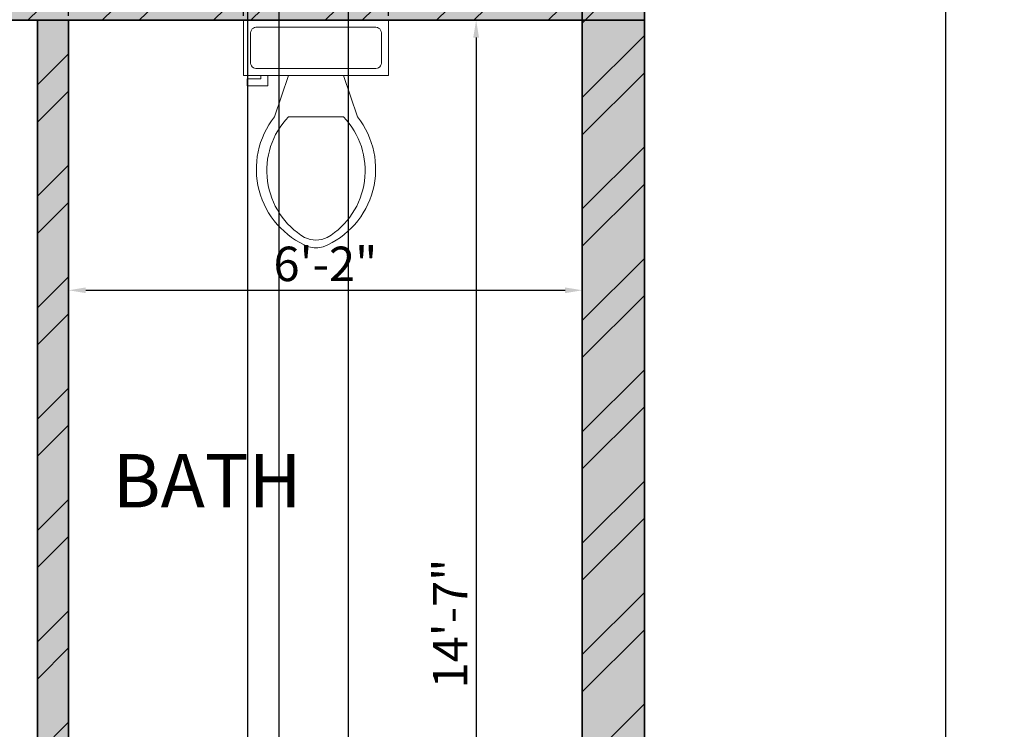
# Model space of a CAD drawing. Units: inches. Extents: x 1804 to 3296, y 909 to 2477.
# Tile 17 of 31: x 2235 to 2378, y 1484 to 1587. Entities that reach past the tile are written whole.
import ezdxf

# ---------------------------------------------------------------- set-up
doc = ezdxf.new("R2010")
doc.units = ezdxf.units.IN
for name, color, linetype, lineweight in [('A-ANNO-DIMS', 2, 'Continuous', 18), ('A-ANNO-TTLB', 156, 'Continuous', 35), ('A-AREA-IDEN', 190, 'Continuous', 18), ('A-FLOR-FIXT', 9, 'Continuous', 18), ('A-WALL-PATT', 10, 'Continuous', 13), ('WALL', 10, 'Continuous', 35)]:
    doc.layers.add(name, color=color, linetype=linetype, lineweight=lineweight)
doc.styles.get("Standard").update_dxf_attribs({"font": 'arial.ttf'})
doc.dimstyles.new('ISO-25', dxfattribs={"dimtxt": 5, "dimasz": 2.5, "dimexe": 1.25, "dimexo": 0.625, "dimtad": 1, "dimdec": 0, "dimlunit": 4, "dimtxsty": 'Standard', "dimcen": 2.5, "dimadec": 0, "dimazin": 0, "dimtfac": 1, "dimtdec": 0, "dimtmove": 0, "dimatfit": 3, "dimfxl": 1, "dimarcsym": 0})
pattern_1 = [(45, (0, 196.207), (-8.08223, 8.08223), []), (45, (5.388, 196.207), (-8.08223, 8.08223), [])]

# ---------------------------------------------------------------- blocks, each defined once
blk = doc.blocks.new('*U4')
for p, q in [((9.5, -6), (9.5, -2)), ((-10, -8.5), (-8, -8.5)), ((-10, -9.5), (-10, -8.5)), ((-8, -8.5), (-8, -8)), ((-7, -8), (-7, -9.5)), ((-4, -8), (-6, -14)), ((4, -8), (6, -14)), ((-7, -9.5), (-10, -9.5)), ((4, -14), (-4, -14))]:
    blk.add_line(p, q)
blk.add_lwpolyline([(10.5, -8), (10.5, 0), (-10.5, 0), (-10.5, -8)], close=True)
for points in [[(8.5, -1), (-8.5, -1)], [(-9.5, -2), (-9.5, -6)], [(-8.5, -7), (8.5, -7)]]:
    blk.add_lwpolyline(points)
for centre, radius, start, end in [((-8.62, -1.88), 0.884, 81.8699, 188.1301), ((8.62, -1.88), 0.884, 351.8699, 98.1301), ((-8.62, -6.12), 0.884, 171.8699, 278.1301), ((8.62, -6.12), 0.884, 261.8699, 8.1301), ((3.52, -21.58), 12.17, 141.4691, 247.9714), ((4.2, -21.82), 11.33, 136.3677, 238.9468), ((-3.52, -21.58), 12.17, 292.0284, 38.5307), ((-4.2, -21.82), 11.33, 301.053, 43.6321), ((0, -27.88), 4, 245.7318, 294.2682), ((0, -29), 4, 254.8605, 285.1395)]:
    blk.add_arc(centre, radius, start, end)
blk = doc.blocks.new('*D12')
at = {"layer": 'A-ANNO-DIMS', "color": 0, "lineweight": -2, "transparency": 16777216}
for p, q in [((2242.06, 1585.8), (2242.06, 1546)), ((2316.54, 1585.8), (2316.54, 1546)), ((2244.56, 1547.25), (2314.04, 1547.25))]:
    blk.add_line(p, q, dxfattribs=at)
at = {"layer": 'A-ANNO-DIMS', "color": 0, "lineweight": 100, "transparency": 16777216}
for points in [[(2244.56, 1547.66), (2244.56, 1546.83), (2242.06, 1547.25)], [(2314.04, 1547.66), (2314.04, 1546.83), (2316.54, 1547.25)]]:
    blk.add_solid(points, dxfattribs=at)
at = {"layer": 'Defpoints', "color": 0, "lineweight": 100, "transparency": 16777216}
for p in [(2242.06, 1586.42), (2316.54, 1586.42), (2316.54, 1547.25)]:
    blk.add_point(p, dxfattribs=at)
at = {"layer": 'A-ANNO-DIMS', "color": 0, "transparency": 16777216, "insert": (2279.3, 1550.43), "char_height": 5, "attachment_point": 5}
blk.add_mtext('6\'-2"', dxfattribs=at)
blk = doc.blocks.new('*D13')
at = {"layer": 'A-ANNO-DIMS', "color": 0, "lineweight": -2, "transparency": 16777216}
for p, q in [((2315.91, 1586.42), (2299.9, 1586.42)), ((2301.15, 1583.92), (2301.15, 1413.85)), ((2315.91, 1411.35), (2299.9, 1411.35))]:
    blk.add_line(p, q, dxfattribs=at)
at = {"layer": 'A-ANNO-DIMS', "color": 0, "lineweight": 100, "transparency": 16777216}
for points in [[(2300.73, 1583.92), (2301.57, 1583.92), (2301.15, 1586.42)], [(2300.73, 1413.85), (2301.57, 1413.85), (2301.15, 1411.35)]]:
    blk.add_solid(points, dxfattribs=at)
at = {"layer": 'Defpoints', "color": 0, "lineweight": 100, "transparency": 16777216}
for p in [(2316.54, 1586.42), (2301.15, 1411.35), (2316.54, 1411.35)]:
    blk.add_point(p, dxfattribs=at)
at = {"layer": 'A-ANNO-DIMS', "color": 0, "transparency": 16777216, "insert": (2298.02, 1498.89), "char_height": 5, "attachment_point": 5, "rotation": 90}
blk.add_mtext('14\'-7"', dxfattribs=at)
blk = doc.blocks.new('*D53')
at = {"layer": 'A-ANNO-DIMS', "color": 0, "lineweight": -2, "transparency": 16777216}
for p, q in [((2326.16, 1793.38), (2370.49, 1793.38)), ((2369.24, 1140.57), (2369.24, 1790.88)), ((2326.16, 1138.07), (2370.49, 1138.07))]:
    blk.add_line(p, q, dxfattribs=at)
at = {"layer": 'A-ANNO-DIMS', "color": 0, "lineweight": 100, "transparency": 16777216}
for points in [[(2368.82, 1790.88), (2369.65, 1790.88), (2369.24, 1793.38)], [(2368.82, 1140.57), (2369.65, 1140.57), (2369.24, 1138.07)]]:
    blk.add_solid(points, dxfattribs=at)
at = {"layer": 'Defpoints', "color": 0, "lineweight": 100, "transparency": 16777216}
for p in [(2325.54, 1793.38), (2369.24, 1793.38), (2325.54, 1138.07)]:
    blk.add_point(p, dxfattribs=at)
at = {"layer": 'A-ANNO-DIMS', "color": 0, "transparency": 16777216, "insert": (2366.03, 1465.72), "char_height": 5, "attachment_point": 5, "rotation": 90}
blk.add_mtext('54\'-7 1/2"', dxfattribs=at)
blk = doc.blocks.new('*D56')
at = {"layer": 'A-ANNO-DIMS', "color": 0, "lineweight": -2, "transparency": 16777216}
for p, q in [((2180.87, 1680.42), (2180.87, 975.89)), ((2268, 1680.42), (2268, 975.89)), ((2183.37, 977.14), (2265.5, 977.14))]:
    blk.add_line(p, q, dxfattribs=at)
at = {"layer": 'A-ANNO-DIMS', "color": 0, "lineweight": 100, "transparency": 16777216}
for points in [[(2183.37, 977.56), (2183.37, 976.72), (2180.87, 977.14)], [(2265.5, 977.56), (2265.5, 976.72), (2268, 977.14)]]:
    blk.add_solid(points, dxfattribs=at)
at = {"layer": 'Defpoints', "color": 0, "lineweight": 100, "transparency": 16777216}
for p in [(2180.87, 1681.04), (2268, 1681.04), (2268, 977.14)]:
    blk.add_point(p, dxfattribs=at)
at = {"layer": 'A-ANNO-DIMS', "color": 0, "transparency": 16777216, "insert": (2224.44, 980.32), "char_height": 5, "attachment_point": 5}
blk.add_mtext('7\'-3"', dxfattribs=at)
blk = doc.blocks.new('*D65')
at = {"layer": 'A-ANNO-DIMS', "color": 0, "lineweight": -2, "transparency": 16777216}
for p, q in [((2282.65, 1466.57), (2282.65, 1874.99)), ((2316.54, 1466.57), (2316.54, 1874.99)), ((2285.15, 1873.74), (2314.04, 1873.74))]:
    blk.add_line(p, q, dxfattribs=at)
at = {"layer": 'A-ANNO-DIMS', "color": 0, "lineweight": 100, "transparency": 16777216}
for points in [[(2285.15, 1874.15), (2285.15, 1873.32), (2282.65, 1873.74)], [(2314.04, 1874.15), (2314.04, 1873.32), (2316.54, 1873.74)]]:
    blk.add_solid(points, dxfattribs=at)
at = {"layer": 'Defpoints', "color": 0, "lineweight": 100, "transparency": 16777216}
for p in [(2316.54, 1873.74), (2282.65, 1465.94), (2316.54, 1465.94)]:
    blk.add_point(p, dxfattribs=at)
at = {"layer": 'A-ANNO-DIMS', "color": 0, "transparency": 16777216, "insert": (2299.6, 1876.91), "char_height": 5, "attachment_point": 5}
blk.add_mtext('2\'-10"', dxfattribs=at)
blk = doc.blocks.new('*D67')
at = {"layer": 'A-ANNO-DIMS', "color": 0, "lineweight": -2, "transparency": 16777216}
for p, q in [((2267.43, 1587.05), (2267.43, 1874.99)), ((2288.43, 1587.05), (2288.43, 1874.99)), ((2269.93, 1873.74), (2285.93, 1873.74))]:
    blk.add_line(p, q, dxfattribs=at)
at = {"layer": 'A-ANNO-DIMS', "color": 0, "lineweight": 100, "transparency": 16777216}
for points in [[(2269.93, 1874.15), (2269.93, 1873.32), (2267.43, 1873.74)], [(2285.93, 1874.15), (2285.93, 1873.32), (2288.43, 1873.74)]]:
    blk.add_solid(points, dxfattribs=at)
at = {"layer": 'Defpoints', "color": 0, "lineweight": 100, "transparency": 16777216}
for p in [(2288.43, 1873.74), (2267.43, 1586.42), (2288.43, 1586.42)]:
    blk.add_point(p, dxfattribs=at)
at = {"layer": 'A-ANNO-DIMS', "color": 0, "transparency": 16777216, "insert": (2277.93, 1876.91), "char_height": 5, "attachment_point": 5}
blk.add_mtext('1\'-9"', dxfattribs=at)
blk = doc.blocks.new('*D68')
at = {"layer": 'A-ANNO-DIMS', "color": 0, "lineweight": -2, "transparency": 16777216}
for p, q in [((2242.06, 1587.05), (2242.06, 1874.99)), ((2267.43, 1587.05), (2267.43, 1874.99)), ((2244.56, 1873.74), (2264.93, 1873.74)), ((2267.43, 1873.74), (2296.2, 1873.74))]:
    blk.add_line(p, q, dxfattribs=at)
at = {"layer": 'A-ANNO-DIMS', "color": 0, "lineweight": 100, "transparency": 16777216}
for points in [[(2244.56, 1874.15), (2244.56, 1873.32), (2242.06, 1873.74)], [(2264.93, 1874.15), (2264.93, 1873.32), (2267.43, 1873.74)]]:
    blk.add_solid(points, dxfattribs=at)
at = {"layer": 'Defpoints', "color": 0, "lineweight": 100, "transparency": 16777216}
for p in [(2267.43, 1873.74), (2242.06, 1586.42), (2267.43, 1586.42)]:
    blk.add_point(p, dxfattribs=at)
at = {"layer": 'A-ANNO-DIMS', "color": 0, "transparency": 16777216, "insert": (2283.07, 1876.95), "char_height": 5, "attachment_point": 5}
blk.add_mtext('2\'-1 1/2"', dxfattribs=at)
blk = doc.blocks.new('*D73')
at = {"layer": 'A-ANNO-DIMS', "color": 0, "lineweight": -2, "transparency": 16777216}
for p, q in [((2272.59, 1272.26), (2272.59, 1874.99)), ((2316.54, 1272.26), (2316.54, 1874.99)), ((2275.09, 1873.74), (2314.04, 1873.74))]:
    blk.add_line(p, q, dxfattribs=at)
at = {"layer": 'A-ANNO-DIMS', "color": 0, "lineweight": 100, "transparency": 16777216}
for points in [[(2275.09, 1874.15), (2275.09, 1873.32), (2272.59, 1873.74)], [(2314.04, 1874.15), (2314.04, 1873.32), (2316.54, 1873.74)]]:
    blk.add_solid(points, dxfattribs=at)
at = {"layer": 'Defpoints', "color": 0, "lineweight": 100, "transparency": 16777216}
for p in [(2316.54, 1873.74), (2272.59, 1271.63), (2316.54, 1271.63)]:
    blk.add_point(p, dxfattribs=at)
at = {"layer": 'A-ANNO-DIMS', "color": 0, "transparency": 16777216, "insert": (2294.56, 1876.92), "char_height": 5, "attachment_point": 5}
blk.add_mtext('3\'-8"', dxfattribs=at)

msp = doc.modelspace()

# ---------------------------------------------------------------- hatches: boundary and pattern name
at = {"layer": 'A-ANNO-TTLB'}
h = msp.add_hatch(color=256, dxfattribs=at)
h.dxf.hatch_style = 1
h.paths.add_polyline_path([(3294.53, 2476.54), (1803.79, 2476.54), (1805.43, 909.47), (3296.17, 909.47)])
h.paths.add_polyline_path([(1811, 914.33), (1812.79, 2467.54), (3285.53, 2467.54), (3283.74, 914.33)], flags=16)
h.paths.add_polyline_path([(1925.58, 1062.77), (1925.58, 1138.07), (1925.58, 1539.88), (1925.58, 1793.38), (1925.58, 1830.04), (2325.54, 1830.04), (2325.54, 1793.38), (2325.54, 1586.42), (2325.54, 1138.07), (2325.54, 1062.77)], flags=0)
h.paths.add_polyline_path([(1997.22, 1029.4), (2008.85, 1037.96), (2008.85, 1020.84)], flags=0)
h.paths.add_polyline_path([(1934.58, 1138.07), (1934.58, 1147.07), (2078.77, 1147.07), (2078.77, 1138.07), (2060.94, 1138.07)], flags=0)
h.paths.add_polyline_path([(1944.35, 1138.07), (1944.35, 1147.07), (2056.05, 1147.07), (2056.05, 1138.07)], flags=0)
h.paths.add_polyline_path([(2222.24, 1037.96), (2233.87, 1029.4), (2222.24, 1020.84)], flags=0)
h.paths.add_polyline_path([(2061.94, 1139.07), (2061.94, 1146.07), (2077.77, 1146.07), (2077.77, 1139.07)], flags=0)
h.paths.add_polyline_path([(2149.58, 1138.07), (2149.58, 1269.44), (2158.58, 1269.44), (2158.58, 1326.69), (2149.58, 1326.69), (2149.58, 1340.94), (2139.6, 1340.94), (2139.6, 1434.25), (2149.58, 1434.25), (2149.58, 1447.36), (2158.58, 1447.36), (2158.58, 1423.87), (2158.58, 1408.06), (2198.46, 1408.06), (2198.46, 1412.56), (2282.65, 1412.56), (2282.65, 1465.94), (2316.54, 1465.94), (2316.54, 1590.92), (2192.86, 1590.92), (2192.86, 1595.3), (2291.17, 1595.3), (2291.17, 1590.92), (2316.54, 1590.92), (2316.54, 1784.38), (2300.24, 1784.38), (2300.24, 1757.47), (2268, 1757.47), (2268, 1681.04), (2180.87, 1681.04), (2180.87, 1757.47), (2148.63, 1757.47), (2148.63, 1784.38), (2119.08, 1784.38), (2119.08, 1585.58), (2114.58, 1585.58), (2114.58, 1784.38), (2064.11, 1784.38), (2046.28, 1784.38), (2046.28, 1760.38), (1958.58, 1760.38), (1958.58, 1664.38), (1934.58, 1664.38), (1934.58, 1784.38), (1934.58, 1793.38), (2046.28, 1793.38), (2064.11, 1793.38), (2119.08, 1793.38), (2230.78, 1793.38), (2230.78, 1784.38), (2268, 1784.38), (2300.24, 1784.38), (2316.54, 1784.38), (2316.54, 1590.92), (2316.54, 1373.73), (2316.54, 1138.07)], flags=0)
h.paths.add_polyline_path([(2209.19, 1166.63), (2209.19, 1175.63), (2158.58, 1175.63), (2209.19, 1223.63), (2209.19, 1231.63), (2183.88, 1231.63), (2183.88, 1301.66), (2242.59, 1301.66), (2242.59, 1326.69), (2316.54, 1326.69), (2272.59, 1271.63), (2272.59, 1223.63), (2316.54, 1175.63), (2272.59, 1175.63), (2272.59, 1166.63)], flags=0)
h.paths.add_polyline_path([(1947.77, 1345.22), (1947.77, 1457.48), (1991.2, 1457.48), (1991.2, 1451.7), (1991.2, 1352.18), (1991.2, 1345.22)], flags=0)
h.paths.add_polyline_path([(2209.19, 1271.63), (2262.59, 1271.63), (2262.59, 1311.85), (2272.59, 1301.66), (2272.59, 1271.63), (2269.92, 1269.63), (2270.59, 1269.63), (2270.59, 1225.63), (2211.19, 1225.63), (2211.19, 1269.63), (2211.86, 1269.63)], flags=0)
h.paths.add_polyline_path([(2000.34, 1378.21), (2000.34, 1429.71), (2025.22, 1429.71), (2025.22, 1378.21)], flags=0)
h.paths.add_polyline_path([(2001.34, 1379.21), (2001.34, 1428.71), (2024.22, 1428.71), (2024.22, 1379.21)], flags=0)
h.paths.add_polyline_path([(2012.34, 1390.21), (2012.34, 1417.71), (2013.22, 1417.71), (2013.22, 1390.21)], flags=0)
h.paths.add_polyline_path([(2237.56, 1331.19), (2237.56, 1340.18), (2238.62, 1340.18), (2238.62, 1386.84), (2241.04, 1386.84), (2242.06, 1386.84), (2242.06, 1408.06), (2316.54, 1331.19)], flags=0)
h.paths.add_polyline_path([(1953.73, 1464.35), (1953.73, 1498.59), (1981.74, 1498.59), (1981.74, 1464.35)], flags=0)
h.paths.add_polyline_path([(1987.63, 1462.08), (1987.63, 1500.95), (2104.07, 1500.95), (2104.07, 1462.08), (2099.27, 1462.08), (1993.6, 1462.08)], flags=0)
h.paths.add_polyline_path([(1956.06, 1481.47, -1), (1979.41, 1481.47, -1)], flags=0)
edge = h.paths.add_edge_path(flags=0)
edge.add_ellipse((2299.53, 1438.37), major_axis=(0.31, 21.36), ratio=0.670333, start_angle=0, end_angle=360)
h.paths.add_polyline_path([(2297.39, 1438.37, -1), (2301.67, 1438.37, -1)], flags=0)
h.paths.add_polyline_path([(2591.54, 1163.23), (2591.54, 1179.38), (2591.54, 1379.68), (2591.54, 1395.84), (2734.5, 1395.84), (2734.5, 1379.68), (2734.5, 1179.38), (2734.5, 1163.23)], flags=0)
h.paths.add_polyline_path([(2592.54, 1164.23), (2592.54, 1166.23), (2733.5, 1166.23), (2733.5, 1164.23)], flags=0)
h.paths.add_polyline_path([(2592.54, 1180.38), (2592.54, 1378.68), (2733.5, 1378.68), (2733.5, 1180.38)], flags=0)
h.paths.add_polyline_path([(2593.54, 1181.38), (2593.54, 1377.68), (2732.5, 1377.68), (2732.5, 1181.38)], flags=0)
h.paths.add_polyline_path([(2594.54, 1182.38), (2594.54, 1376.68), (2731.5, 1376.68), (2731.5, 1182.38)], flags=0)
h.paths.add_polyline_path([(1936.95, 1697.46), (1936.95, 1736.46), (1955.41, 1736.46), (1955.41, 1697.46)], flags=0)
h.paths.add_polyline_path([(1938.48, 1718.36), (1938.48, 1734.92), (1953.65, 1734.92), (1953.65, 1718.36)], flags=0)
h.paths.add_polyline_path([(1944.75, 1726.64, -1), (1947.37, 1726.64, -1)], flags=0)
h.paths.add_polyline_path([(2592.54, 1394.84), (2733.5, 1394.84), (2733.5, 1392.84), (2592.54, 1392.84)], flags=0)
h.paths.add_polyline_path([(1976.61, 1762.5), (1976.61, 1781.44), (2012.79, 1781.44), (2012.79, 1762.5)], flags=0)
h.paths.add_polyline_path([(1979.57, 1771.97, -1), (1991.39, 1771.97, -1)], flags=0)
h.paths.add_polyline_path([(1995.36, 1771.97, -1), (2007.18, 1771.97, -1)], flags=0)
h.paths.add_polyline_path([(2251.51, 1744.53), (2268, 1730.05), (2251.51, 1730.05)], flags=0)
h.paths.add_polyline_path([(2047.28, 1785.38), (2047.28, 1792.38), (2063.11, 1792.38), (2063.11, 1785.38)], flags=0)
h.paths.add_polyline_path([(2155.08, 1770.92, -1), (2174.42, 1770.92, -1)], flags=0)
h.paths.add_polyline_path([(2188.59, 1758.27), (2188.59, 1772.81), (2222.3, 1772.81), (2222.3, 1758.27)], flags=0)
h.paths.add_polyline_path([(2223.97, 1758.27), (2223.97, 1772.81), (2257.68, 1772.81), (2257.68, 1758.27)], flags=0)
h.paths.add_polyline_path([(2274.45, 1770.92, -1), (2293.8, 1770.92, -1)], flags=0)
h.paths.add_polyline_path([(2591.54, 1582.09), (2591.54, 1782.39), (2734.5, 1782.39), (2734.5, 1582.09)], flags=0)
h.paths.add_polyline_path([(2592.54, 1583.09), (2592.54, 1781.39), (2733.5, 1781.39), (2733.5, 1583.09)], flags=0)
h.paths.add_polyline_path([(2593.54, 1584.09), (2593.54, 1780.39), (2732.5, 1780.39), (2732.5, 1584.09)], flags=0)
h.paths.add_polyline_path([(2594.54, 1585.09), (2594.54, 1779.39), (2731.5, 1779.39), (2731.5, 1585.09)], flags=0)
h.paths.add_polyline_path([(1922.17, 1978.79), (1922.17, 2295.08), (1922.17, 2296.08), (2115.67, 2296.08), (2115.67, 2384.31), (2115.67, 2385.31), (2322.12, 2385.31), (2323.12, 2385.31), (2323.12, 1979.79), (2323.12, 1978.79), (1923.17, 1978.79)], flags=0)
h.paths.add_polyline_path([(1922.17, 1978.79), (1922.17, 2051.31), (1922.17, 2214.86), (1922.17, 2296.08), (2115.67, 2296.08), (2115.67, 2385.31), (2323.12, 2385.31), (2323.12, 2280.42), (2323.12, 1978.79), (2115.67, 1978.79)], flags=0)
h.paths.add_polyline_path([(1923.17, 1979.79), (1923.17, 2050.31), (2115.67, 2050.31), (2115.67, 2051.31), (1923.17, 2051.31), (1923.17, 2213.86), (1923.17, 2214.86), (1923.17, 2295.08), (1990.02, 2295.08), (1990.02, 2214.86), (1991.02, 2214.86), (1991.02, 2295.08), (2115.67, 2295.08), (2115.67, 1979.79), (2116.67, 1979.79), (2116.67, 2304.18), (2116.67, 2384.31), (2322.12, 2384.31), (2322.12, 2280.42), (2322.12, 1979.79), (2115.67, 1979.79)], flags=0)
h.paths.add_polyline_path([(2972.46, 1192.5), (2972.46, 1196.92), (2995.47, 1196.92), (2995.47, 1255.47), (2995.09, 1255.47), (2987.42, 1249.39), (2980.08, 1255.47), (2978.05, 1255.47), (2978.05, 1257.24), (2995.47, 1257.24), (2995.47, 1261.58), (3015.37, 1261.58), (3015.37, 1333.28), (3015.37, 1414.4), (3032.82, 1414.4), (3032.82, 1333.28), (3032.82, 1261.58), (3052.66, 1261.58), (3052.66, 1255.47), (3079.86, 1255.47), (3078.72, 1254.57), (3081.47, 1252.29), (3078.56, 1249.99), (3075.81, 1252.26), (3072.57, 1249.69), (3070.36, 1251.52), (3067.67, 1249.39), (3060.34, 1255.47), (3052.66, 1255.47), (3052.66, 1196.92), (3054.58, 1196.92), (3074, 1196.92), (3074, 1192.5), (3052.66, 1192.5), (2995.47, 1192.5)], flags=0)
h.paths.add_polyline_path([(2490.75, 1979.27), (2490.75, 1980.27), (2596.87, 1980.27), (2596.87, 2051.8), (2596.87, 2052.8), (2596.87, 2216.35), (2596.87, 2297.57), (2717.32, 2297.57), (2710.57, 2305.62), (2724.07, 2305.62), (2717.32, 2297.57), (2782.37, 2297.57), (2782.37, 2395.8), (3006.82, 2395.8), (3006.82, 1981.27), (3093.73, 1981.27), (3093.73, 1980.27), (3047.51, 1980.27), (3046.37, 1979.37), (3049.11, 1977.1), (3046.2, 1974.79), (3043.46, 1977.07), (3040.21, 1974.49), (3038, 1976.32), (3035.32, 1974.2), (3027.98, 1980.27), (2871.83, 1980.27), (2871.83, 1981.27), (2791.37, 1981.27), (2791.37, 2050.8), (2597.87, 2050.8), (2597.87, 1980.27), (2597.87, 1979.27), (2546.27, 1979.27), (2545.12, 1978.37), (2547.87, 1976.1), (2544.96, 1973.79), (2542.22, 1976.07), (2538.97, 1973.49), (2536.76, 1975.32), (2534.07, 1973.2), (2526.74, 1979.27)], flags=0)
h.paths.add_polyline_path([(2597.87, 2051.8), (2606.87, 2051.8), (2606.87, 2258.39), (2597.87, 2258.39), (2597.87, 2296.57), (2606.87, 2296.57), (2606.87, 2262.39), (2782.37, 2262.39), (2782.37, 2296.57), (2790.37, 2296.57), (2790.37, 2262.39), (2791.37, 2262.39), (2791.37, 2305.67), (2791.37, 2385.8), (2996.82, 2385.8), (2996.82, 2339.85), (3006.82, 2339.85), (3006.82, 2250.12), (2997.82, 2250.12), (2997.82, 1981.27), (2996.82, 1981.27), (2872.83, 1981.27), (2872.83, 1991.8), (2871.83, 1991.8), (2871.83, 2050.8), (2790.37, 2050.8), (2597.87, 2050.8)], flags=0)
h.paths.add_polyline_path([(2179.93, 2153.92), (2179.93, 2353.97), (2259.98, 2353.97), (2259.98, 2153.92)], flags=0)
h.paths.add_polyline_path([(2180.93, 2154.92), (2180.93, 2352.97), (2258.98, 2352.97), (2258.98, 2154.92)], flags=0)
h.paths.add_polyline_path([(2960.87, 1608.49), (2960.87, 1753.62), (3070.9, 1753.62), (3070.9, 1608.49)], flags=0)
h.paths.add_polyline_path([(2961.87, 1609.49), (2961.87, 1752.62), (3069.9, 1752.62), (3069.9, 1609.49)], flags=0)
h.paths.add_polyline_path([(2962.87, 1610.49), (2962.87, 1751.62), (3068.9, 1751.62), (3068.9, 1610.49)], flags=0)
h.paths.add_polyline_path([(2963.87, 1611.49), (2963.87, 1750.62), (3067.9, 1750.62), (3067.9, 1611.49)], flags=0)
h.paths.add_polyline_path([(2782.37, 2051.8), (2782.37, 2216.32), (2791.37, 2216.32), (2791.37, 2051.8), (2872.83, 2051.8), (2872.83, 2068.56), (2884.67, 2068.56), (2884.67, 2085.33), (2896.51, 2085.33), (2896.51, 2102.09), (2908.36, 2102.09), (2908.36, 2118.85), (2920.2, 2118.85), (2920.2, 2135.62), (2932.05, 2135.62), (2932.05, 2145.3), (2925.08, 2145.3), (2925.08, 2203.2), (2996.82, 2203.2), (2996.82, 2145.3), (2953.82, 2145.3), (2872.83, 2051.8), (2790.37, 2051.8)], flags=0)
h.paths.add_polyline_path([(2717.32, 2238.65), (2710.57, 2246.7), (2724.07, 2246.7)], flags=0)
h.paths.add_polyline_path([(2003.09, 1122.79), (2017.16, 1122.79), (2017.16, 1138.74), (2003.09, 1138.74)], flags=8)
h.paths.add_polyline_path([(2174.76, 1792.72), (2188.83, 1792.72), (2188.83, 1808.66), (2174.76, 1808.66)], flags=8)
h.paths.add_polyline_path([(1987.95, 1792.51), (2002.02, 1792.51), (2002.02, 1808.45), (1987.95, 1808.45)], flags=8)
h.paths.add_polyline_path([(2148.79, 1289.26), (2160.46, 1289.26), (2160.46, 1305.2), (2148.79, 1305.2)], flags=8)
h.paths.add_polyline_path([(2115.36, 1133.57), (2127.04, 1133.57), (2127.04, 1149.51), (2115.36, 1149.51)], flags=8)
h.paths.add_polyline_path([(2237.58, 1421.48), (2249.25, 1421.48), (2249.25, 1437.43), (2237.58, 1437.43)], flags=8)
h.paths.add_polyline_path([(2134.99, 1584.32), (2146.66, 1584.32), (2146.66, 1600.26), (2134.99, 1600.26)], flags=8)
h.paths.add_polyline_path([(2101.95, 1557.31), (2113.62, 1557.31), (2113.62, 1573.25), (2101.95, 1573.25)], flags=8)
h.paths.add_polyline_path([(2937.85, 1156.77), (3120.41, 1156.77), (3120.41, 1185.72), (2937.85, 1185.72)], flags=8)
h.paths.add_polyline_path([(2980.71, 1786.71), (3050.06, 1786.71), (3050.06, 1802.66), (2980.71, 1802.66)], flags=8)
h.paths.add_polyline_path([(2869.28, 1661.96), (2938.62, 1661.96), (2938.62, 1690.8), (2869.28, 1690.8)], flags=8)
h.paths.add_polyline_path([(3092.27, 1674.86), (3161.62, 1674.86), (3161.62, 1690.8), (3092.27, 1690.8)], flags=8)
h.paths.add_polyline_path([(2980.71, 1674.86), (3050.06, 1674.86), (3050.06, 1690.8), (2980.71, 1690.8)], flags=8)
h.paths.add_polyline_path([(2649.07, 1678.23), (2674.53, 1678.23), (2674.53, 1714.76), (2649.07, 1714.76)], flags=8)
h.paths.add_polyline_path([(2530.84, 1981.63), (2549.13, 1981.63), (2549.13, 1997.57), (2530.84, 1997.57)], flags=8)
h.paths.add_polyline_path([(3031.29, 1981.77), (3049.58, 1981.77), (3049.58, 1997.71), (3031.29, 1997.71)], flags=8)
h.paths.add_polyline_path([(2715.38, 1911.9), (2851.54, 1911.9), (2851.54, 1940.85), (2715.38, 1940.85)], flags=8)
h.paths.add_polyline_path([(2015.23, 1927.36), (2205.42, 1927.36), (2205.42, 1956.3), (2015.23, 1956.3)], flags=8)
h.paths.add_polyline_path([(2671.84, 2057.84), (2702.75, 2057.84), (2702.75, 2073.79), (2671.84, 2073.79)], flags=8)
h.paths.add_polyline_path([(2678.5, 2316.52), (2765.26, 2316.52), (2765.26, 2332.46), (2678.5, 2332.46)], flags=8)
h.paths.add_polyline_path([(2678.48, 2271.96), (2736.41, 2271.96), (2736.41, 2287.9), (2678.48, 2287.9)], flags=8)
h.paths.add_polyline_path([(2019.2, 972.79), (2243.21, 972.79), (2243.21, 1001.74), (2019.2, 1001.74)], flags=8)
h.paths.add_polyline_path([(2097.06, 1021.56), (2132.16, 1021.56), (2132.16, 1037.51), (2097.06, 1037.51)], flags=8)
h.paths.add_polyline_path([(2182.47, 1360.48), (2207.35, 1360.48), (2207.35, 1376.42), (2182.47, 1376.42)], flags=8)
h.paths.add_polyline_path([(2261.12, 1361.77), (2295.01, 1361.77), (2295.01, 1377.71), (2261.12, 1377.71)], flags=8)
h.paths.add_polyline_path([(2245.75, 1511.51), (2278.44, 1511.51), (2278.44, 1527.46), (2245.75, 1527.46)], flags=8)
h.paths.add_polyline_path([(1991.16, 1296.29), (2060.51, 1296.29), (2060.51, 1312.23), (1991.16, 1312.23)], flags=8)
h.paths.add_polyline_path([(2187, 1651.35), (2246.71, 1651.35), (2246.71, 1667.29), (2187, 1667.29)], flags=8)
h.paths.add_polyline_path([(1976.49, 1684.81), (2068.63, 1684.81), (2068.63, 1700.76), (1976.49, 1700.76)], flags=8)
at = {"layer": 'A-WALL-PATT'}
h = msp.add_hatch(color=256, dxfattribs=at)
h.dxf.hatch_style = 1
h.paths.add_polyline_path([(2119.08, 1544.38), (1925.58, 1544.38), (1925.58, 1539.88), (2119.08, 1539.88)])
h.paths.add_polyline_path([(2119.08, 1545.58), (2114.58, 1545.58), (2114.58, 1544.38), (2119.08, 1544.38)])
h.paths.add_polyline_path([(1965.87, 1658.79), (1965.87, 1679.09), (1955.57, 1679.09), (1955.57, 1658.79)], flags=9)
h.paths.add_polyline_path([(2293.18, 1677.29), (2293.18, 1697.58), (2282.88, 1697.58), (2282.88, 1677.29)], flags=9)
h.paths.add_polyline_path([(2271.13, 1545.23), (2287.53, 1545.23), (2287.53, 1555.53), (2271.13, 1555.53)], flags=9)
h.paths.add_polyline_path([(2303.26, 1488.52), (2303.26, 1508.82), (2292.95, 1508.82), (2292.95, 1488.52)], flags=9)
h.paths.add_polyline_path([(2271.13, 1393.15), (2287.53, 1393.15), (2287.53, 1403.45), (2271.13, 1403.45)], flags=9)
h.paths.add_polyline_path([(2306.48, 1361.45), (2306.48, 1377.86), (2296.18, 1377.86), (2296.18, 1361.45)], flags=9)
h.paths.add_polyline_path([(2174.54, 1361.45), (2174.54, 1377.86), (2164.23, 1377.86), (2164.23, 1361.45)], flags=9)
h.paths.add_polyline_path([(1968.21, 1333.34), (1968.21, 1353.64), (1957.91, 1353.64), (1957.91, 1333.34)], flags=9)
h.paths.add_polyline_path([(2003.09, 1122.79), (2017.16, 1122.79), (2017.16, 1138.74), (2003.09, 1138.74)], flags=9)
h.paths.add_polyline_path([(2174.76, 1792.72), (2188.83, 1792.72), (2188.83, 1808.66), (2174.76, 1808.66)], flags=9)
h.paths.add_polyline_path([(1987.95, 1792.51), (2002.02, 1792.51), (2002.02, 1808.45), (1987.95, 1808.45)], flags=9)
h.paths.add_polyline_path([(2148.79, 1289.26), (2160.46, 1289.26), (2160.46, 1305.2), (2148.79, 1305.2)], flags=9)
h.paths.add_polyline_path([(2115.36, 1133.57), (2127.04, 1133.57), (2127.04, 1149.51), (2115.36, 1149.51)], flags=9)
h.paths.add_polyline_path([(2237.58, 1421.48), (2249.25, 1421.48), (2249.25, 1437.43), (2237.58, 1437.43)], flags=9)
h.paths.add_polyline_path([(2134.99, 1584.32), (2146.66, 1584.32), (2146.66, 1600.26), (2134.99, 1600.26)], flags=9)
h.paths.add_polyline_path([(2101.95, 1557.31), (2113.62, 1557.31), (2113.62, 1573.25), (2101.95, 1573.25)], flags=9)
h.paths.add_polyline_path([(2937.85, 1156.77), (3120.41, 1156.77), (3120.41, 1185.72), (2937.85, 1185.72)], flags=9)
h.paths.add_polyline_path([(2980.71, 1786.71), (3050.06, 1786.71), (3050.06, 1802.66), (2980.71, 1802.66)], flags=9)
h.paths.add_polyline_path([(2869.28, 1661.96), (2938.62, 1661.96), (2938.62, 1690.8), (2869.28, 1690.8)], flags=9)
h.paths.add_polyline_path([(3092.27, 1674.86), (3161.62, 1674.86), (3161.62, 1690.8), (3092.27, 1690.8)], flags=9)
h.paths.add_polyline_path([(2980.71, 1674.86), (3050.06, 1674.86), (3050.06, 1690.8), (2980.71, 1690.8)], flags=9)
h.paths.add_polyline_path([(2649.07, 1678.23), (2674.53, 1678.23), (2674.53, 1714.76), (2649.07, 1714.76)], flags=9)
h.paths.add_polyline_path([(2530.84, 1981.63), (2549.13, 1981.63), (2549.13, 1997.57), (2530.84, 1997.57)], flags=9)
h.paths.add_polyline_path([(3031.29, 1981.77), (3049.58, 1981.77), (3049.58, 1997.71), (3031.29, 1997.71)], flags=9)
h.paths.add_polyline_path([(2715.38, 1911.9), (2851.54, 1911.9), (2851.54, 1940.85), (2715.38, 1940.85)], flags=9)
h.paths.add_polyline_path([(2015.23, 1927.36), (2205.42, 1927.36), (2205.42, 1956.3), (2015.23, 1956.3)], flags=9)
h.paths.add_polyline_path([(2671.84, 2057.84), (2702.75, 2057.84), (2702.75, 2073.79), (2671.84, 2073.79)], flags=9)
h.paths.add_polyline_path([(2678.5, 2316.52), (2765.26, 2316.52), (2765.26, 2332.46), (2678.5, 2332.46)], flags=9)
h.paths.add_polyline_path([(2678.48, 2271.96), (2736.41, 2271.96), (2736.41, 2287.9), (2678.48, 2287.9)], flags=9)
h.paths.add_polyline_path([(2019.2, 972.79), (2243.21, 972.79), (2243.21, 1001.74), (2019.2, 1001.74)], flags=9)
h.paths.add_polyline_path([(2097.06, 1021.56), (2132.16, 1021.56), (2132.16, 1037.51), (2097.06, 1037.51)], flags=9)
h.paths.add_polyline_path([(2182.47, 1360.48), (2207.35, 1360.48), (2207.35, 1376.42), (2182.47, 1376.42)], flags=9)
h.paths.add_polyline_path([(2261.12, 1361.77), (2295.01, 1361.77), (2295.01, 1377.71), (2261.12, 1377.71)], flags=9)
h.paths.add_polyline_path([(2245.75, 1511.51), (2278.44, 1511.51), (2278.44, 1527.46), (2245.75, 1527.46)], flags=9)
h.paths.add_polyline_path([(1991.16, 1296.29), (2060.51, 1296.29), (2060.51, 1312.23), (1991.16, 1312.23)], flags=9)
h.paths.add_polyline_path([(2187, 1651.35), (2246.71, 1651.35), (2246.71, 1667.29), (2187, 1667.29)], flags=9)
h.paths.add_polyline_path([(1976.49, 1684.81), (2068.63, 1684.81), (2068.63, 1700.76), (1976.49, 1700.76)], flags=9)
h = msp.add_hatch(color=256, dxfattribs=at)
h.dxf.hatch_style = 1
h.paths.add_polyline_path([(2149.58, 1147.07), (2141.21, 1147.07), (2141.21, 1144.07), (2141.21, 1138.07), (2149.58, 1138.07)])
h.paths.add_polyline_path([(2101.21, 1144.07, -0.01877), (2101.32, 1147.07), (2078.77, 1147.07), (2078.77, 1138.07), (2101.21, 1138.07)])
h.paths.add_polyline_path([(2060.94, 1147.07), (2056.05, 1147.07), (2056.05, 1138.07), (2060.94, 1138.07)])
h.paths.add_polyline_path([(1944.35, 1147.07), (1934.58, 1147.07), (1934.58, 1138.07), (1944.35, 1138.07)])
h.paths.add_polyline_path([(2158.58, 1269.44), (2149.58, 1269.44), (2149.58, 1138.07), (2158.58, 1138.07)])
h.paths.add_polyline_path([(2003.09, 1122.79), (2017.16, 1122.79), (2017.16, 1138.74), (2003.09, 1138.74)], flags=9)
h.paths.add_polyline_path([(2174.76, 1792.72), (2188.83, 1792.72), (2188.83, 1808.66), (2174.76, 1808.66)], flags=9)
h.paths.add_polyline_path([(1987.95, 1792.51), (2002.02, 1792.51), (2002.02, 1808.45), (1987.95, 1808.45)], flags=9)
h.paths.add_polyline_path([(2148.79, 1289.26), (2160.46, 1289.26), (2160.46, 1305.2), (2148.79, 1305.2)], flags=9)
h.paths.add_polyline_path([(2115.36, 1133.57), (2127.04, 1133.57), (2127.04, 1149.51), (2115.36, 1149.51)], flags=9)
h.paths.add_polyline_path([(2237.58, 1421.48), (2249.25, 1421.48), (2249.25, 1437.43), (2237.58, 1437.43)], flags=9)
h.paths.add_polyline_path([(2134.99, 1584.32), (2146.66, 1584.32), (2146.66, 1600.26), (2134.99, 1600.26)], flags=9)
h.paths.add_polyline_path([(2101.95, 1557.31), (2113.62, 1557.31), (2113.62, 1573.25), (2101.95, 1573.25)], flags=9)
h.paths.add_polyline_path([(2937.85, 1156.77), (3120.41, 1156.77), (3120.41, 1185.72), (2937.85, 1185.72)], flags=9)
h.paths.add_polyline_path([(2980.71, 1786.71), (3050.06, 1786.71), (3050.06, 1802.66), (2980.71, 1802.66)], flags=9)
h.paths.add_polyline_path([(2869.28, 1661.96), (2938.62, 1661.96), (2938.62, 1690.8), (2869.28, 1690.8)], flags=9)
h.paths.add_polyline_path([(3092.27, 1674.86), (3161.62, 1674.86), (3161.62, 1690.8), (3092.27, 1690.8)], flags=9)
h.paths.add_polyline_path([(2980.71, 1674.86), (3050.06, 1674.86), (3050.06, 1690.8), (2980.71, 1690.8)], flags=9)
h.paths.add_polyline_path([(2649.07, 1678.23), (2674.53, 1678.23), (2674.53, 1714.76), (2649.07, 1714.76)], flags=9)
h.paths.add_polyline_path([(2530.84, 1981.63), (2549.13, 1981.63), (2549.13, 1997.57), (2530.84, 1997.57)], flags=9)
h.paths.add_polyline_path([(3031.29, 1981.77), (3049.58, 1981.77), (3049.58, 1997.71), (3031.29, 1997.71)], flags=9)
h.paths.add_polyline_path([(2715.38, 1911.9), (2851.54, 1911.9), (2851.54, 1940.85), (2715.38, 1940.85)], flags=9)
h.paths.add_polyline_path([(2015.23, 1927.36), (2205.42, 1927.36), (2205.42, 1956.3), (2015.23, 1956.3)], flags=9)
h.paths.add_polyline_path([(2671.84, 2057.84), (2702.75, 2057.84), (2702.75, 2073.79), (2671.84, 2073.79)], flags=9)
h.paths.add_polyline_path([(2678.5, 2316.52), (2765.26, 2316.52), (2765.26, 2332.46), (2678.5, 2332.46)], flags=9)
h.paths.add_polyline_path([(2678.48, 2271.96), (2736.41, 2271.96), (2736.41, 2287.9), (2678.48, 2287.9)], flags=9)
h.paths.add_polyline_path([(2019.2, 972.79), (2243.21, 972.79), (2243.21, 1001.74), (2019.2, 1001.74)], flags=9)
h.paths.add_polyline_path([(2097.06, 1021.56), (2132.16, 1021.56), (2132.16, 1037.51), (2097.06, 1037.51)], flags=9)
h.paths.add_polyline_path([(2182.47, 1360.48), (2207.35, 1360.48), (2207.35, 1376.42), (2182.47, 1376.42)], flags=9)
h.paths.add_polyline_path([(2261.12, 1361.77), (2295.01, 1361.77), (2295.01, 1377.71), (2261.12, 1377.71)], flags=9)
h.paths.add_polyline_path([(2245.75, 1511.51), (2278.44, 1511.51), (2278.44, 1527.46), (2245.75, 1527.46)], flags=9)
h.paths.add_polyline_path([(1991.16, 1296.29), (2060.51, 1296.29), (2060.51, 1312.23), (1991.16, 1312.23)], flags=9)
h.paths.add_polyline_path([(2187, 1651.35), (2246.71, 1651.35), (2246.71, 1667.29), (2187, 1667.29)], flags=9)
h.paths.add_polyline_path([(1976.49, 1684.81), (2068.63, 1684.81), (2068.63, 1700.76), (1976.49, 1700.76)], flags=9)
h = msp.add_hatch(color=256, dxfattribs=at)
h.dxf.hatch_style = 1
h.paths.add_polyline_path([(2158.58, 1275.49), (2155.29, 1275.49), (2149.58, 1275.49), (2149.58, 1269.44), (2158.58, 1269.44)])
h.paths.add_polyline_path([(2158.58, 1326.69), (2149.58, 1326.69), (2149.58, 1319.33), (2155.29, 1319.33), (2158.58, 1319.33)])
h.paths.add_polyline_path([(2158.58, 1402.2), (2158.58, 1423.87), (2158.58, 1447.36), (2149.58, 1447.36), (2149.58, 1423.87), (2149.58, 1340.94), (2149.58, 1326.69), (2158.58, 1326.69), (2158.58, 1354.23)])
h.paths.add_polyline_path([(1965.87, 1658.79), (1965.87, 1679.09), (1955.57, 1679.09), (1955.57, 1658.79)], flags=9)
h.paths.add_polyline_path([(2293.18, 1677.29), (2293.18, 1697.58), (2282.88, 1697.58), (2282.88, 1677.29)], flags=9)
h.paths.add_polyline_path([(2271.13, 1545.23), (2287.53, 1545.23), (2287.53, 1555.53), (2271.13, 1555.53)], flags=9)
h.paths.add_polyline_path([(2303.26, 1488.52), (2303.26, 1508.82), (2292.95, 1508.82), (2292.95, 1488.52)], flags=9)
h.paths.add_polyline_path([(2271.13, 1393.15), (2287.53, 1393.15), (2287.53, 1403.45), (2271.13, 1403.45)], flags=9)
h.paths.add_polyline_path([(2306.48, 1361.45), (2306.48, 1377.86), (2296.18, 1377.86), (2296.18, 1361.45)], flags=9)
h.paths.add_polyline_path([(2189.9, 1340.62), (2206.31, 1340.62), (2206.31, 1350.92), (2189.9, 1350.92)], flags=9)
h.paths.add_polyline_path([(2174.54, 1361.45), (2174.54, 1377.86), (2164.23, 1377.86), (2164.23, 1361.45)], flags=9)
h.paths.add_polyline_path([(2304.24, 1240.8), (2304.24, 1261.09), (2293.94, 1261.09), (2293.94, 1240.8)], flags=9)
h.paths.add_polyline_path([(2227.19, 1188.73), (2247.49, 1188.73), (2247.49, 1199.03), (2227.19, 1199.03)], flags=9)
h.paths.add_polyline_path([(2181.93, 1144.21), (2181.93, 1160.62), (2171.63, 1160.62), (2171.63, 1144.21)], flags=9)
h.paths.add_polyline_path([(1968.21, 1333.34), (1968.21, 1353.64), (1957.91, 1353.64), (1957.91, 1333.34)], flags=9)
h.paths.add_polyline_path([(2029.78, 1203.53), (2053.95, 1203.53), (2053.95, 1213.83), (2029.78, 1213.83)], flags=9)
h.paths.add_polyline_path([(2576.51, 1671.88), (2576.51, 1692.17), (2566.21, 1692.17), (2566.21, 1671.88)], flags=9)
h.paths.add_polyline_path([(2566.99, 1269.67), (2566.99, 1289.96), (2556.68, 1289.96), (2556.68, 1269.67)], flags=9)
h.paths.add_polyline_path([(2581.85, 1269.17), (2581.85, 1289.46), (2571.54, 1289.46), (2571.54, 1269.17)], flags=9)
h.paths.add_polyline_path([(2650.71, 1409.75), (2674.89, 1409.75), (2674.89, 1420.05), (2650.71, 1420.05)], flags=9)
h.paths.add_polyline_path([(2003.09, 1122.79), (2017.16, 1122.79), (2017.16, 1138.74), (2003.09, 1138.74)], flags=9)
h.paths.add_polyline_path([(2174.76, 1792.72), (2188.83, 1792.72), (2188.83, 1808.66), (2174.76, 1808.66)], flags=9)
h.paths.add_polyline_path([(1987.95, 1792.51), (2002.02, 1792.51), (2002.02, 1808.45), (1987.95, 1808.45)], flags=9)
h.paths.add_polyline_path([(2148.79, 1289.26), (2160.46, 1289.26), (2160.46, 1305.2), (2148.79, 1305.2)], flags=9)
h.paths.add_polyline_path([(2115.36, 1133.57), (2127.04, 1133.57), (2127.04, 1149.51), (2115.36, 1149.51)], flags=9)
h.paths.add_polyline_path([(2237.58, 1421.48), (2249.25, 1421.48), (2249.25, 1437.43), (2237.58, 1437.43)], flags=9)
h.paths.add_polyline_path([(2134.99, 1584.32), (2146.66, 1584.32), (2146.66, 1600.26), (2134.99, 1600.26)], flags=9)
h.paths.add_polyline_path([(2101.95, 1557.31), (2113.62, 1557.31), (2113.62, 1573.25), (2101.95, 1573.25)], flags=9)
h.paths.add_polyline_path([(2937.85, 1156.77), (3120.41, 1156.77), (3120.41, 1185.72), (2937.85, 1185.72)], flags=9)
h.paths.add_polyline_path([(2980.71, 1786.71), (3050.06, 1786.71), (3050.06, 1802.66), (2980.71, 1802.66)], flags=9)
h.paths.add_polyline_path([(2869.28, 1661.96), (2938.62, 1661.96), (2938.62, 1690.8), (2869.28, 1690.8)], flags=9)
h.paths.add_polyline_path([(3092.27, 1674.86), (3161.62, 1674.86), (3161.62, 1690.8), (3092.27, 1690.8)], flags=9)
h.paths.add_polyline_path([(2980.71, 1674.86), (3050.06, 1674.86), (3050.06, 1690.8), (2980.71, 1690.8)], flags=9)
h.paths.add_polyline_path([(2649.07, 1678.23), (2674.53, 1678.23), (2674.53, 1714.76), (2649.07, 1714.76)], flags=9)
h.paths.add_polyline_path([(2530.84, 1981.63), (2549.13, 1981.63), (2549.13, 1997.57), (2530.84, 1997.57)], flags=9)
h.paths.add_polyline_path([(3031.29, 1981.77), (3049.58, 1981.77), (3049.58, 1997.71), (3031.29, 1997.71)], flags=9)
h.paths.add_polyline_path([(2715.38, 1911.9), (2851.54, 1911.9), (2851.54, 1940.85), (2715.38, 1940.85)], flags=9)
h.paths.add_polyline_path([(2015.23, 1927.36), (2205.42, 1927.36), (2205.42, 1956.3), (2015.23, 1956.3)], flags=9)
h.paths.add_polyline_path([(2671.84, 2057.84), (2702.75, 2057.84), (2702.75, 2073.79), (2671.84, 2073.79)], flags=9)
h.paths.add_polyline_path([(2678.5, 2316.52), (2765.26, 2316.52), (2765.26, 2332.46), (2678.5, 2332.46)], flags=9)
h.paths.add_polyline_path([(2678.48, 2271.96), (2736.41, 2271.96), (2736.41, 2287.9), (2678.48, 2287.9)], flags=9)
h.paths.add_polyline_path([(2019.2, 972.79), (2243.21, 972.79), (2243.21, 1001.74), (2019.2, 1001.74)], flags=9)
h.paths.add_polyline_path([(2097.06, 1021.56), (2132.16, 1021.56), (2132.16, 1037.51), (2097.06, 1037.51)], flags=9)
h.paths.add_polyline_path([(2182.47, 1360.48), (2207.35, 1360.48), (2207.35, 1376.42), (2182.47, 1376.42)], flags=9)
h.paths.add_polyline_path([(2261.12, 1361.77), (2295.01, 1361.77), (2295.01, 1377.71), (2261.12, 1377.71)], flags=9)
h.paths.add_polyline_path([(2245.75, 1511.51), (2278.44, 1511.51), (2278.44, 1527.46), (2245.75, 1527.46)], flags=9)
h.paths.add_polyline_path([(1991.16, 1296.29), (2060.51, 1296.29), (2060.51, 1312.23), (1991.16, 1312.23)], flags=9)
h.paths.add_polyline_path([(2187, 1651.35), (2246.71, 1651.35), (2246.71, 1667.29), (2187, 1667.29)], flags=9)
h.paths.add_polyline_path([(1976.49, 1684.81), (2068.63, 1684.81), (2068.63, 1700.76), (1976.49, 1700.76)], flags=9)
h = msp.add_hatch(dxfattribs=at)
h.set_pattern_fill('ANSI32', color=256, scale=1.2)
h.set_pattern_definition(pattern_1)
h.paths.add_polyline_path([(1934.58, 1784.38), (1934.58, 1793.38), (1925.58, 1793.38), (1925.58, 1539.88), (2119.08, 1539.88), (2119.08, 1545.58), (2114.58, 1545.58), (2114.58, 1544.38), (1934.58, 1544.38)])
h.paths.add_polyline_path([(2114.58, 1793.38), (2064.11, 1793.38), (2064.11, 1784.38), (2114.58, 1784.38)], flags=17)
h.paths.add_polyline_path([(2325.54, 1793.38), (2230.78, 1793.38), (2230.78, 1784.38), (2268, 1784.38), (2300.24, 1784.38), (2316.54, 1784.38), (2316.54, 1590.92), (2316.54, 1586.42), (2325.54, 1586.42)])
h.paths.add_polyline_path([(1944.35, 1147.07), (1934.58, 1147.07), (1934.58, 1138.07), (1944.35, 1138.07)])
h.paths.add_polyline_path([(2101.21, 1144.07, -0.01877), (2101.32, 1147.07), (2078.77, 1147.07), (2078.77, 1138.07), (2101.21, 1138.07)])
h.paths.add_polyline_path([(1934.58, 1539.88), (1925.58, 1539.88), (1925.58, 1138.07), (1934.58, 1138.07), (1934.58, 1147.07)])
h.paths.add_polyline_path([(2325.54, 1586.42), (2316.54, 1586.42), (2316.54, 1373.73), (2316.54, 1138.07), (2325.54, 1138.07), (2325.54, 1228.97)])
h.paths.add_polyline_path([(2158.58, 1423.87), (2158.58, 1447.36), (2149.58, 1447.36), (2149.58, 1423.87), (2149.58, 1340.94), (2149.58, 1326.69), (2158.58, 1326.69), (2158.58, 1354.23), (2158.58, 1402.2)])
h.paths.add_polyline_path([(2316.54, 1412.56), (2282.65, 1412.56), (2273.09, 1412.56), (2273.09, 1408.06), (2316.54, 1408.06)])
h.paths.add_polyline_path([(2273.09, 1412.56), (2242.06, 1412.56), (2242.06, 1408.06), (2273.09, 1408.06)])
h.paths.add_polyline_path([(2237.56, 1412.56), (2198.46, 1412.56), (2198.46, 1408.06), (2237.56, 1408.06)])
h.paths.add_polyline_path([(2242.06, 1408.06), (2237.56, 1408.06), (2237.56, 1386.84), (2242.06, 1386.84)])
h.paths.add_polyline_path([(2242.06, 1412.56), (2237.56, 1412.56), (2237.56, 1408.06), (2242.06, 1408.06)])
h.paths.add_polyline_path([(2158.58, 1269.44), (2149.58, 1269.44), (2149.58, 1138.07), (2158.58, 1138.07)])
h.paths.add_polyline_path([(2149.58, 1147.07), (2141.21, 1147.07), (2141.21, 1144.07), (2141.21, 1138.07), (2149.58, 1138.07)])
h.paths.add_polyline_path([(2272.59, 1175.63), (2209.19, 1175.63), (2209.19, 1166.63), (2272.59, 1166.63)])
h.paths.add_polyline_path([(2237.56, 1446.21), (2242.06, 1446.21), (2242.06, 1586.42), (2237.56, 1586.42)])
h.paths.add_polyline_path([(2242.06, 1414.58), (2237.56, 1414.58), (2237.56, 1412.56), (2242.06, 1412.56)])
h = msp.add_hatch(color=256, dxfattribs=at)
h.dxf.hatch_style = 1
h.paths.add_polyline_path([(2114.58, 1793.38), (2064.11, 1793.38), (2064.11, 1784.38), (2114.58, 1784.38)])
h.paths.add_polyline_path([(2119.08, 1793.38), (2114.58, 1793.38), (2114.58, 1585.58), (2119.08, 1585.58)])
h.paths.add_polyline_path([(2325.54, 1793.38), (2230.78, 1793.38), (2230.78, 1784.38), (2268, 1784.38), (2316.54, 1784.38), (2316.54, 1590.92), (2316.54, 1586.42), (2325.54, 1586.42)])
h.paths.add_polyline_path([(2316.54, 1331.19), (2158.58, 1331.19), (2158.58, 1326.69), (2316.54, 1326.69)])
h.paths.add_polyline_path([(2242.06, 1408.06), (2237.56, 1408.06), (2237.56, 1386.84), (2242.06, 1386.84)])
h.paths.add_polyline_path([(2242.06, 1412.56), (2237.56, 1412.56), (2237.56, 1408.06), (2242.06, 1408.06)])
h.paths.add_polyline_path([(2237.56, 1412.56), (2198.46, 1412.56), (2198.46, 1408.06), (2237.56, 1408.06)])
h.paths.add_polyline_path([(2273.09, 1412.56), (2242.06, 1412.56), (2242.06, 1408.06), (2273.09, 1408.06)])
h.paths.add_polyline_path([(2316.54, 1412.56), (2282.65, 1412.56), (2273.09, 1412.56), (2273.09, 1408.06), (2316.54, 1408.06)])
h.paths.add_polyline_path([(2325.54, 1586.42), (2316.54, 1586.42), (2316.54, 1373.73), (2316.54, 1138.07), (2325.54, 1138.07), (2325.54, 1228.97)])
h.paths.add_polyline_path([(2272.59, 1175.63), (2209.19, 1175.63), (2209.19, 1166.63), (2272.59, 1166.63)])
h = msp.add_hatch(dxfattribs=at)
h.set_pattern_fill('ANSI32', color=256, scale=1.2)
h.set_pattern_definition(pattern_1)
h.paths.add_polyline_path([(2161.83, 1590.92), (2161.83, 1586.42), (2316.54, 1586.42), (2316.54, 1590.92)])
h = msp.add_hatch(color=256, dxfattribs=at)
h.dxf.hatch_style = 1
h.paths.add_polyline_path([(2316.54, 1590.92), (2161.83, 1590.92), (2161.83, 1586.42), (2316.54, 1586.42)])
h = msp.add_hatch(color=256, dxfattribs=at)
h.dxf.hatch_style = 1
h.paths.add_polyline_path([(2242.06, 1586.42), (2237.56, 1586.42), (2237.56, 1446.21), (2242.06, 1446.21)])

# ---------------------------------------------------------------- linework, layer by layer
at = {"layer": 'WALL'}
for p, q in [((2325.54, 1793.38), (2325.54, 1586.42)), ((2316.54, 1590.92), (2316.54, 1373.73)), ((2325.54, 1586.42), (2161.83, 1586.42)), ((2237.56, 1586.42), (2237.56, 1446.21)), ((2237.56, 1446.21), (2237.56, 1586.42)), ((2242.06, 1586.42), (2242.06, 1446.21)), ((2325.54, 1586.42), (2325.54, 1138.07))]:
    msp.add_line(p, q, dxfattribs=at)
for points in [[(2161.83, 1586.42), (2316.54, 1586.42), (2316.54, 1590.92), (2161.83, 1590.92)], [(2237.56, 1446.21), (2242.06, 1446.21), (2242.06, 1586.42), (2237.56, 1586.42)]]:
    msp.add_lwpolyline(points, close=True, dxfattribs=at)

# ---------------------------------------------------------------- block references
at = {"layer": 'A-FLOR-FIXT'}
msp.add_blockref('*U4', (2277.93, 1586.42), dxfattribs=at)

# ---------------------------------------------------------------- texts
at = {"layer": 'A-AREA-IDEN', "insert": (2248.47, 1523.48), "char_height": 7.737, "attachment_point": 1}
msp.add_mtext_dynamic_manual_height_columns('BATH', width=163.3261, gutter_width=38.69, heights=[0], dxfattribs=at)

# ---------------------------------------------------------------- dimensions: what is measured, and where the dimension line sits
at = {"layer": 'A-ANNO-DIMS'}
for base, p1, p2, override, picture, middle in [((2267.43, 1873.74), (2242.06, 1586.42), (2267.43, 1586.42), {"dimdec": 1, "dimlfac": 1, "dimrnd": 0, "dimzin": 1, "dimdsep": 46, "dimlunit": 4, "dimfrac": 2}, '*D68', (2283.07, 1876.95)), ((2288.43, 1873.74), (2267.43, 1586.42), (2288.43, 1586.42), {"dimdec": 1, "dimlfac": 1, "dimrnd": 0, "dimzin": 1, "dimdsep": 46, "dimlunit": 4, "dimfrac": 2}, '*D67', (2277.93, 1876.91)), ((2316.5375, 1873.7362), (2272.5886, 1271.6342), (2316.5375, 1271.6342), {"dimdec": 1, "dimlfac": 1, "dimrnd": 0, "dimzin": 1, "dimdsep": 46, "dimlunit": 4, "dimfrac": 2}, '*D73', (2294.563, 1876.9158)), ((2316.54, 1873.74), (2282.65, 1465.94), (2316.54, 1465.94), {"dimdec": 1, "dimlfac": 1, "dimrnd": 0, "dimzin": 1, "dimdsep": 46, "dimlunit": 4, "dimfrac": 2}, '*D65', (2299.6, 1876.91)), ((2268, 977.14), (2180.87, 1681.04), (2268, 1681.04), {"dimdec": 1, "dimlfac": 1, "dimrnd": 0, "dimzin": 1, "dimdsep": 46, "dimlunit": 4, "dimfrac": 2}, '*D56', (2224.44, 980.32)), ((2316.54, 1547.25), (2242.06, 1586.42), (2316.54, 1586.42), {"dimclrd": 0, "dimclre": 0, "dimclrt": 0}, '*D12', (2279.3, 1550.43))]:
    dim = msp.add_linear_dim(base=base, p1=p1, p2=p2, dimstyle='ISO-25', override=override, dxfattribs=at)
    dim.commit()
    dim.dimension.update_dxf_attribs({"geometry": picture, "text_midpoint": middle})
for base, p1, p2, override, picture, middle in [((2369.24, 1793.38), (2325.54, 1138.07), (2325.54, 1793.38), {"dimdec": 1, "dimlfac": 1, "dimrnd": 0, "dimzin": 1, "dimdsep": 46, "dimlunit": 4, "dimfrac": 2}, '*D53', (2366.03, 1465.72)), ((2301.15, 1411.35), (2316.54, 1586.42), (2316.54, 1411.35), {"dimclrd": 0, "dimclre": 0, "dimclrt": 0}, '*D13', (2298.02, 1498.89))]:
    dim = msp.add_linear_dim(base=base, p1=p1, p2=p2, angle=90, dimstyle='ISO-25', override=override, dxfattribs=at)
    dim.commit()
    dim.dimension.update_dxf_attribs({"geometry": picture, "text_midpoint": middle})

doc.saveas('drawing.dxf')
